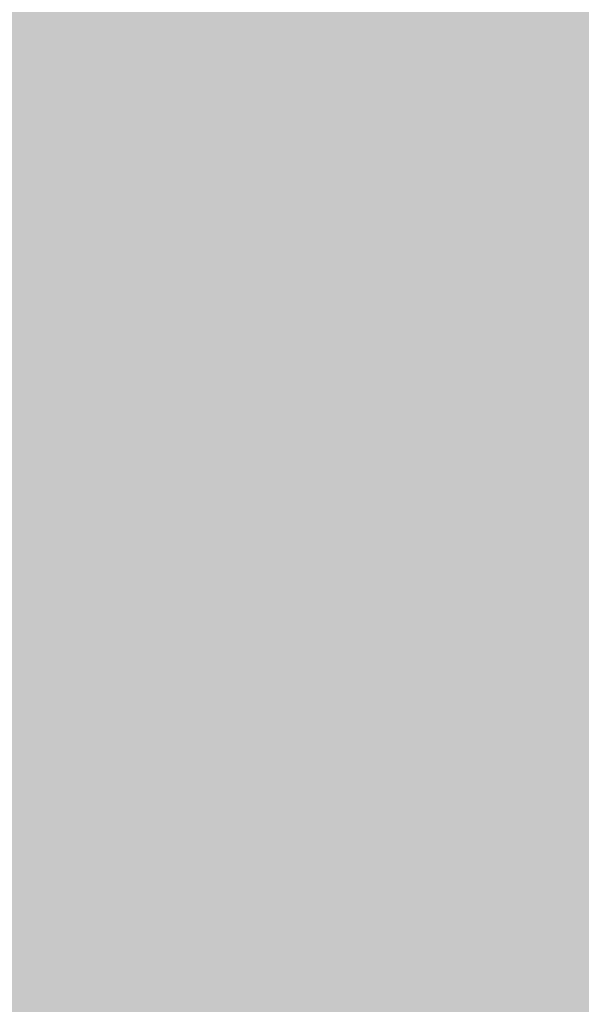
# Model space of a CAD drawing. Units: inches. Extents: x 2083 to 3317, y 1141 to 2115.
# Tile 171 of 256: x 3126.94671 to 3126.95594, y 1263.27402 to 1263.29018. Entities that reach past the tile are written whole.
import ezdxf

# ---------------------------------------------------------------- set-up
doc = ezdxf.new("R2010")
doc.units = ezdxf.units.IN
doc.layers.add('A-ANNO-DIMS', color=2, linetype='Continuous', lineweight=18)
doc.layers.add('A-WALL-PATT', color=251, linetype='Continuous', lineweight=13, true_color=0x636466)
doc.styles.get("Standard").update_dxf_attribs({"font": 'arial.ttf'})
doc.dimstyles.new('ISO-25', dxfattribs={"dimtxt": 12, "dimasz": 12, "dimexe": 1.25, "dimexo": 0.625, "dimtad": 1, "dimlunit": 3, "dimtxsty": 'Standard', "dimcen": 2.5, "dimadec": 0, "dimazin": 0, "dimtfac": 1, "dimtmove": 0, "dimatfit": 3, "dimfxl": 1, "dimarcsym": 0})

# ---------------------------------------------------------------- blocks, each defined once
blk = doc.blocks.new('*D26')
at = {"layer": 'A-ANNO-DIMS', "color": 0, "lineweight": -2, "transparency": 16777216}
for p, q in [((3088.985844, 1274.915092), (3088.985844, 1270.951963)), ((3111.240037, 1274.915092), (3111.240037, 1270.951963)), ((3076.985844, 1272.201963), (2840.262447, 1272.201963)), ((3111.240037, 1272.201963), (3088.985844, 1272.201963)), ((3123.240037, 1272.201963), (3135.240037, 1272.201963))]:
    blk.add_line(p, q, dxfattribs=at)
at = {"layer": 'A-ANNO-DIMS', "color": 0, "transparency": 16777216}
for points in [[(3076.985844, 1274.201963), (3076.985844, 1270.201963), (3088.985844, 1272.201963)], [(3123.240037, 1274.201963), (3123.240037, 1270.201963), (3111.240037, 1272.201963)]]:
    blk.add_solid(points, dxfattribs=at)
at = {"layer": 'Defpoints', "color": 0, "transparency": 16777216}
for p in [(3088.985844, 1275.540092), (3111.240037, 1275.540092), (3088.985844, 1272.201963)]:
    blk.add_point(p, dxfattribs=at)
at = {"layer": 'A-ANNO-DIMS', "color": 0, "transparency": 16777216, "insert": (2952.624146, 1279.031602), "char_height": 12, "attachment_point": 5}
blk.add_mtext('NIGHTSTAND 1\'-10 1/2" TYP.', dxfattribs=at)
blk = doc.blocks.new('*D27')
at = {"layer": 'A-ANNO-DIMS', "color": 0, "lineweight": -2, "transparency": 16777216}
for p, q in [((3114.578165, 1309.794285), (3114.578165, 1321.794285)), ((3111.865037, 1297.794285), (3115.828165, 1297.794285)), ((3114.578165, 1297.794285), (3114.578165, 1275.540092)), ((3111.865037, 1275.540092), (3115.828165, 1275.540092)), ((3114.578165, 1263.540092), (3114.578165, 1140.988591))]:
    blk.add_line(p, q, dxfattribs=at)
at = {"layer": 'A-ANNO-DIMS', "color": 0, "transparency": 16777216}
for points in [[(3112.578165, 1309.794285), (3116.578165, 1309.794285), (3114.578165, 1297.794285)], [(3112.578165, 1263.540092), (3116.578165, 1263.540092), (3114.578165, 1275.540092)]]:
    blk.add_solid(points, dxfattribs=at)
at = {"layer": 'Defpoints', "color": 0, "transparency": 16777216}
for p in [(3111.240037, 1297.794285), (3111.240037, 1275.540092), (3114.578165, 1275.540092)]:
    blk.add_point(p, dxfattribs=at)
at = {"layer": 'A-ANNO-DIMS', "color": 0, "transparency": 16777216, "insert": (3107.748527, 1196.264342), "char_height": 12, "attachment_point": 5, "rotation": 90}
blk.add_mtext('1\'-10 1/2" TYP.', dxfattribs=at)

msp = doc.modelspace()

# ---------------------------------------------------------------- hatches: boundary and pattern name
at = {"layer": 'A-WALL-PATT'}
h = msp.add_hatch(color=256, dxfattribs=at)
h.dxf.hatch_style = 1
h.paths.add_polyline_path([(3126.959783, 2020.76136), (2748.959783, 2020.76136), (2604.959783, 2020.76136), (2226.959783, 2020.76136), (2226.959783, 1702.76136), (2466.959783, 1702.76136), (2466.959783, 1582.76136), (2418.959783, 1582.76136), (2418.959783, 1477.76136), (2226.959783, 1477.76136), (2226.959783, 1263.26136), (2544.959783, 1263.26136), (2544.959783, 1411.76136), (2604.959783, 1411.76136), (2685.959783, 1411.76136), (2685.959783, 1420.76136), (2604.959783, 1420.76136), (2604.959783, 1573.76136), (2604.959783, 1702.76136), (2604.959783, 2011.76136), (2748.959783, 2011.76136), (2748.959783, 1702.76136), (2862.959783, 1702.76136), (2862.959783, 1621.76136), (2871.959783, 1621.76136), (2871.959783, 1702.76136), (2883.959783, 1702.76136), (2883.959783, 1706.939459, -0.026459), (2883.959783, 1711.76136), (2757.959783, 1711.76136), (2757.959783, 1807.76136), (2787.959783, 1807.76136), (2787.959783, 1812.26136), (2757.959783, 1812.26136), (2757.959783, 2011.76136), (2877.959783, 2011.76136), (2877.959783, 1812.26136), (2847.959783, 1812.26136), (2847.959783, 1807.76136), (2889.835742, 1807.76136), (2889.835742, 1812.26136), (2882.459783, 1812.26136), (2882.459783, 2011.76136), (3117.959783, 2011.76136), (3117.959783, 1812.26136), (2937.835742, 1812.26136), (2937.835742, 1807.76136), (2995.709783, 1807.76136), (2995.709783, 1796.117666), (3000.209783, 1796.117666), (3000.209783, 1807.76136), (3117.959783, 1807.76136), (3117.959783, 1711.76136), (3000.209783, 1711.76136), (3000.209783, 1760.117666), (2998.572705, 1760.117666, -0.020711), (2995.709783, 1760.117666), (2995.709783, 1711.76136), (2931.959783, 1711.76136), (2931.959783, 1702.76136), (3126.959783, 1702.76136)])
h.paths.add_polyline_path([(2471.459783, 2011.76136), (2471.459783, 1810.01136), (2462.716936, 1810.01136), (2462.716936, 1805.51136), (2505.959783, 1805.51136), (2505.959783, 1810.01136), (2475.959783, 1810.01136), (2475.959783, 2011.76136), (2595.959783, 2011.76136), (2595.959783, 1810.01136), (2565.959783, 1810.01136), (2565.959783, 1805.51136), (2595.959783, 1805.51136), (2595.959783, 1711.76136), (2235.959783, 1711.76136), (2235.959783, 1805.51136), (2353.709783, 1805.51136), (2353.709783, 1796.054162), (2358.209783, 1796.054162), (2358.209783, 1805.51136), (2414.716936, 1805.51136), (2414.716936, 1810.01136), (2235.959783, 1810.01136), (2235.959783, 2011.76136)], flags=16)
h.paths.add_polyline_path([(2270.204734, 1994.610008), (2270.204734, 1970.610008), (2246.204734, 1970.610008), (2246.204734, 1994.610008)], flags=0)
edge = h.paths.add_edge_path(flags=0)
edge.add_ellipse((2332.027391, 1899.798176), major_axis=(-3.042994, 3.042994), ratio=0.16825245, start_angle=-161.332166, end_angle=-156.307114, ccw=False)
edge.add_ellipse((2333.082037, 1898.74353), major_axis=(-1.054646, 1.054646), ratio=0.4535321, start_angle=-123.371019, end_angle=-94.159107)
edge = h.paths.add_edge_path(flags=0)
edge.add_ellipse((2332.027391, 1968.87629), major_axis=(3.042994, 3.042994), ratio=0.16825245, start_angle=18.667834, end_angle=23.692886)
edge.add_spline(control_points=[(2332.925596, 1970.691105), (2332.226768, 1970.3361), (2330.893709, 1969.658905), (2328.41308, 1970.932138), (2327.203934, 1967.748712), (2324.709596, 1969.955589), (2322.532822, 1967.012354), (2320.012846, 1971.295812), (2317.680308, 1968.157845), (2316.040526, 1967.102047), (2315.426904, 1966.809602)], knot_values=[0, 0, 0, 0, 2.267059, 4.324559, 6.685584, 8.878641, 11.121502, 14.300359, 17.755284, 19.732645, 19.732645, 19.732645, 19.732645], degree=3, periodic=0)
edge.add_ellipse((2332.027391, 1968.87629), major_axis=(3.042994, 3.042994), ratio=0.16825245, start_angle=18.667834, end_angle=23.692886, ccw=False)
edge.add_ellipse((2333.082037, 1969.930936), major_axis=(1.054646, 1.054646), ratio=0.4535321, start_angle=56.628981, end_angle=85.840893, ccw=False)
edge = h.paths.add_edge_path(flags=0)
edge.add_spline(control_points=[(2296.428287, 1967.987908), (2293.627804, 1965.336314), (2287.703624, 1959.727094), (2299.74386, 1949.995699), (2294.532591, 1935.668528), (2290.573228, 1920.603512), (2293.394124, 1909.973691), (2296.185407, 1904.966543)], knot_values=[0.099185, 0.099185, 0.099185, 0.099185, 0.345301, 0.619822, 0.982653, 1.386093, 1.810555, 1.810555, 1.810555, 1.810555], degree=3, periodic=0)
edge.add_spline(control_points=[(2296.185407, 1904.966543), (2297.383582, 1902.6193), (2298.000969, 1901.949312), (2298.55297, 1901.468155)], knot_values=[0.006246, 0.006246, 0.006246, 0.006246, 0.055476, 0.055476, 0.055476, 0.055476], degree=3, periodic=0)
edge.add_spline(control_points=[(2298.55297, 1901.468155), (2297.258612, 1900.923224), (2295.225294, 1900.232126), (2293.060229, 1900.614205), (2292.101423, 1900.788415), (2292.089578, 1900.790568)], knot_values=[0.312835, 0.312835, 0.312835, 0.312835, 0.40178, 0.474987, 0.475903, 0.475903, 0.475903, 0.475903], degree=3, periodic=0)
edge.add_arc((2292.793646, 1904.664109), 3.937008, 215.420897, 259.698179, ccw=False)
edge.add_spline(control_points=[(2289.585314, 1902.382304), (2289.476652, 1902.535087), (2289.36848, 1902.688035), (2289.260865, 1902.84117)], knot_values=[0.102872, 0.102872, 0.102872, 0.102872, 0.116896, 0.116896, 0.116896, 0.116896], degree=3, periodic=0)
edge.add_spline(control_points=[(2289.260865, 1902.84117), (2288.686604, 1902.550192), (2287.640048, 1902.019902), (2285.881337, 1901.873954), (2283.852972, 1901.504352), (2281.719987, 1899.710538), (2278.466991, 1899.492942), (2276.157136, 1901.883202), (2272.258953, 1899.804071), (2267.777605, 1901.843183), (2262.243882, 1900.184033), (2257.414927, 1901.782061), (2254.318374, 1900.72612), (2253.178285, 1900.337343)], knot_values=[0, 0, 0, 0, 1.907977, 3.477176, 5.261074, 7.972851, 11.680248, 13.717921, 16.939592, 22.789562, 27.502503, 33.595215, 37.145618, 37.145618, 37.145618, 37.145618], degree=3, periodic=0)
edge.add_line((2253.178285, 1900.337343), (2250.24424, 1902.84117))
edge.add_line((2250.24424, 1902.84117), (2250.24424, 1965.833296))
edge.add_line((2250.24424, 1965.833296), (2253.178285, 1968.337123))
edge.add_spline(control_points=[(2253.178285, 1968.337123), (2254.318374, 1967.948346), (2257.414927, 1966.892405), (2262.243882, 1968.490433), (2267.777605, 1966.831283), (2271.52673, 1968.537217), (2273.875914, 1967.828289), (2274.206701, 1967.727642)], knot_values=[0, 0, 0, 0, 0.09018, 0.244935, 0.364644, 0.513233, 0.537855, 0.537855, 0.537855, 0.537855], degree=3, periodic=0)
edge.add_arc((2274.352887, 1963.793349), 3.937008, 72.051134, 92.127949, ccw=False)
edge.add_arc((2281.296933, 1985.230003), 18.596298, 252.0511336, 288.5657217)
edge.add_arc((2292.316717, 1956.02888), 12.646081, 71.0267879, 113.7782184, ccw=False)
edge = h.paths.add_edge_path(flags=0)
edge.add_spline(control_points=[(2274.899415, 1951.856195), (2275.066156, 1951.616592), (2275.232687, 1951.376588), (2275.397987, 1951.135855)], knot_values=[1.409916, 1.409916, 1.409916, 1.409916, 1.43159, 1.43159, 1.43159, 1.43159], degree=3, periodic=0)
edge.add_spline(control_points=[(2275.397987, 1951.135855), (2275.792106, 1950.561885), (2276.179231, 1949.983774), (2276.545546, 1949.397103)], knot_values=[1.358238, 1.358238, 1.358238, 1.358238, 1.409916, 1.409916, 1.409916, 1.409916], degree=3, periodic=0)
edge.add_line((2276.545546, 1949.397103), (2277.437289, 1947.862185))
edge.add_spline(control_points=[(2277.437289, 1947.862185), (2276.303834, 1945.673115), (2274.639698, 1942.426882), (2274.631615, 1938.0939), (2272.799124, 1930.85155), (2274.356426, 1943.897046), (2275.947681, 1947.923356), (2276.545546, 1949.397103)], knot_values=[0.005632, 0.005632, 0.005632, 0.005632, 0.186014, 0.266002, 0.357087, 0.59639, 0.739732, 0.739732, 0.739732, 0.739732], degree=3, periodic=0)
edge.add_spline(control_points=[(2276.545546, 1949.397103), (2276.179231, 1949.983774), (2275.792106, 1950.561885), (2275.397987, 1951.135855)], knot_values=[1.358238, 1.358238, 1.358238, 1.358238, 1.409916, 1.409916, 1.409916, 1.409916], degree=3, periodic=0)
edge.add_spline(control_points=[(2275.397987, 1951.135855), (2274.9425, 1950.080452), (2274.20776, 1948.025272), (2273.934602, 1944.851477), (2272.468534, 1937.627489), (2273.466216, 1945.696466), (2274.700615, 1951.059472), (2274.899415, 1951.856195)], knot_values=[0.104364, 0.104364, 0.104364, 0.104364, 0.189636, 0.269624, 0.36071, 0.600013, 0.644622, 0.644622, 0.644622, 0.644622], degree=3, periodic=0)
h.paths.add_polyline_path([(2269.167514, 1963.127573, -0.357527), (2268.170633, 1960.97637, -0.092561), (2268.170633, 1939.436325, -0.357527), (2269.167514, 1937.285122, -0.357527), (2267.01631, 1938.282002, -0.164785), (2254.685581, 1938.282002, -0.357527), (2252.534378, 1937.285122, -0.357527), (2253.531259, 1939.436325, -0.092561), (2253.531259, 1960.97637, -0.357527), (2252.534378, 1963.127573, -0.357527), (2254.685581, 1962.130692, -0.164785), (2267.01631, 1962.130692, -0.357527)], flags=0)
h.paths.add_polyline_path([(2248.874068, 1967.8018), (2248.874068, 1957.02771), (2249.457783, 1957.02771), (2249.457783, 1911.646756), (2248.874068, 1911.646756), (2248.874068, 1900.872666), (2246.511863, 1900.872666, 0.197327), (2244.149658, 1902.456873), (2244.149658, 1966.217592, 0.197327), (2246.511863, 1967.8018)], flags=0)
h.paths.add_polyline_path([(2269.167514, 1931.389344, -0.357527), (2268.170633, 1929.238141, -0.092561), (2268.170633, 1907.698096, -0.357527), (2269.167514, 1905.546893, -0.357527), (2267.01631, 1906.543774, -0.164785), (2254.685581, 1906.543774, -0.357527), (2252.534378, 1905.546893, -0.357527), (2253.531259, 1907.698096, -0.092561), (2253.531259, 1929.238141, -0.357527), (2252.534378, 1931.389344, -0.357527), (2254.685581, 1930.392463, -0.164785), (2267.01631, 1930.392463, -0.357527)], flags=0)
edge = h.paths.add_edge_path(flags=0)
edge.add_spline(control_points=[(2276.196858, 1906.723702), (2276.168144, 1909.028928), (2276.114049, 1913.371852), (2270.598417, 1924.924978), (2273.905175, 1919.012779), (2275.921711, 1916.262063), (2275.47457, 1912.402149), (2277.257874, 1910.380621), (2276.696044, 1908.225036), (2276.646218, 1906.813023), (2276.617825, 1906.008407)], knot_values=[0, 0, 0, 0, 8.61026, 16.221274, 18.843057, 23.804898, 27.440828, 29.356102, 31.203478, 33.650687, 33.650687, 33.650687, 33.650687], degree=3, periodic=0)
edge.add_spline(control_points=[(2276.617825, 1906.008407), (2276.623313, 1905.624144), (2276.497738, 1904.628661), (2275.441779, 1903.854725), (2274.937314, 1903.08045), (2274.85908, 1902.84117)], knot_values=[0.156488, 0.156488, 0.156488, 0.156488, 0.184398, 0.231376, 0.250598, 0.250598, 0.250598, 0.250598], degree=3, periodic=0)
edge.add_line((2274.85908, 1902.84117), (2276.50598, 1902.84117))
edge.add_spline(control_points=[(2276.50598, 1902.84117), (2276.788308, 1903.08494), (2277.665071, 1904.125196), (2278.249538, 1904.340738), (2277.653872, 1908.527387), (2278.15567, 1906.227808), (2278.100464, 1905.285948), (2278.846675, 1904.069005), (2277.856785, 1903.414948), (2277.874191, 1902.99105), (2277.903562, 1902.84117)], knot_values=[0.059574, 0.059574, 0.059574, 0.059574, 0.080753, 0.103741, 0.16972, 0.176036, 0.207137, 0.240474, 0.262341, 0.27366, 0.27366, 0.27366, 0.27366], degree=3, periodic=0)
edge.add_line((2277.903562, 1902.84117), (2280.029825, 1902.84117))
edge.add_spline(control_points=[(2280.029825, 1902.84117), (2279.888221, 1903.088398), (2279.499257, 1903.981551), (2280.152284, 1905.939349), (2278.103615, 1909.657757), (2279.762395, 1907.185285), (2280.3279, 1904.874861), (2280.485109, 1903.48959), (2281.463269, 1903.249432), (2281.758343, 1902.936497), (2281.834036, 1902.84117)], knot_values=[0.013856, 0.013856, 0.013856, 0.013856, 0.034874, 0.088867, 0.107879, 0.126738, 0.158714, 0.193757, 0.217487, 0.226722, 0.226722, 0.226722, 0.226722], degree=3, periodic=0)
edge.add_spline(control_points=[(2281.834036, 1902.84117), (2281.787535, 1902.826703), (2281.647022, 1902.782988), (2281.395527, 1902.85949), (2281.088077, 1902.985242), (2280.720683, 1903.060902), (2280.333451, 1903.025726), (2280.124767, 1902.898879), (2280.029825, 1902.84117)], knot_values=[0, 0, 0, 0, 0.14413, 0.435517, 0.749276, 1.153046, 1.548371, 1.878348, 1.878348, 1.878348, 1.878348], degree=3, periodic=0)
edge.add_line((2280.029825, 1902.84117), (2277.903562, 1902.84117))
edge.add_spline(control_points=[(2277.903562, 1902.84117), (2277.892855, 1902.795855), (2277.865396, 1902.679637), (2277.607479, 1902.687483), (2277.27405, 1902.8007), (2276.837921, 1902.619775), (2276.583807, 1902.789261), (2276.50598, 1902.84117)], knot_values=[0, 0, 0, 0, 0.127189, 0.326199, 0.628009, 1.24357, 1.515331, 1.515331, 1.515331, 1.515331], degree=3, periodic=0)
edge.add_line((2276.50598, 1902.84117), (2274.85908, 1902.84117))
edge.add_spline(control_points=[(2274.85908, 1902.84117), (2274.814437, 1902.898587), (2274.72513, 1903.013446), (2274.493477, 1903.118968), (2274.244285, 1902.960539), (2273.937121, 1903.184942), (2273.614039, 1902.983143), (2273.408316, 1902.883045), (2273.322254, 1902.84117)], knot_values=[0, 0, 0, 0, 0.21843, 0.436957, 0.687977, 0.990379, 1.398396, 1.69185, 1.69185, 1.69185, 1.69185], degree=3, periodic=0)
edge.add_spline(control_points=[(2273.322254, 1902.84117), (2273.61674, 1903.445692), (2274.273998, 1904.538253), (2276.027239, 1904.573702), (2276.206963, 1906.583637), (2276.196858, 1906.723702)], knot_values=[0.012227, 0.012227, 0.012227, 0.012227, 0.059472, 0.106218, 0.134458, 0.134458, 0.134458, 0.134458], degree=3, periodic=0)
h.paths.add_polyline_path([(2270.776054, 1897.789828), (2270.776054, 1873.789828), (2246.776054, 1873.789828), (2246.776054, 1897.789828)], flags=0)
h.paths.add_polyline_path([(2353.709783, 1760.005059), (2353.709783, 1760.054162), (2358.209783, 1760.054162, -0.033729)], flags=0)
h.paths.add_polyline_path([(2321.819119, 1737.529186), (2341.995327, 1737.529186, -0.414214), (2343.203273, 1736.321241), (2343.203273, 1721.020596, -0.414214), (2341.995327, 1719.812651), (2321.819119, 1719.812651, -0.414214), (2320.611173, 1721.020596), (2320.611173, 1736.321241, -0.414214)], flags=0)
h.paths.add_polyline_path([(2324.23501, 1736.321241), (2339.579436, 1736.321241, -0.414214), (2341.995327, 1733.905349), (2341.995327, 1725.44973, -0.414214), (2339.579436, 1723.033839), (2333.680588, 1723.033839), (2333.845317, 1722.045467, -0.870646), (2335.425399, 1721.825893, -0.767327), (2333.922694, 1721.423245), (2331.291024, 1721.423245, -0.767327), (2329.788319, 1721.825893, -0.870646), (2331.368401, 1722.045467), (2331.53313, 1723.033839), (2324.23501, 1723.033839, -0.414214), (2321.819119, 1725.44973), (2321.819119, 1733.905349, -0.414214)], flags=0)
h.paths.add_polyline_path([(2570.483789, 1928.615444), (2589.683789, 1928.615444), (2590.168829, 1928.615444), (2590.168829, 1904.993397), (2570.483789, 1904.993397)], flags=0)
h.paths.add_polyline_path([(2574.447324, 1927.263822, -1), (2572.828836, 1927.263822, -1)], flags=0)
h.paths.add_polyline_path([(2573.089867, 1926.940877), (2573.925032, 1927.776042), (2574.147743, 1927.553332), (2573.312577, 1926.718166)], flags=0)
h.paths.add_polyline_path([(2578.779065, 1919.729618, -1), (2571.591663, 1919.729618, -1)], flags=0)
h.paths.add_polyline_path([(2578.385364, 1919.729618, -1), (2571.985364, 1919.729618, -1)], flags=0)
h.paths.add_polyline_path([(2331.595764, 1729.476216, -1), (2333.617954, 1729.476216, -1)], flags=0)
h.paths.add_polyline_path([(2578.034228, 1927.263822, -1), (2576.41574, 1927.263822, -1)], flags=0)
h.paths.add_polyline_path([(2576.688851, 1927.531089), (2576.911562, 1927.753799), (2577.746728, 1926.918634), (2577.524017, 1926.695923)], flags=0)
h.paths.add_polyline_path([(2578.139065, 1909.859539, -1), (2572.231663, 1909.859539, -1)], flags=0)
h.paths.add_polyline_path([(2577.745364, 1909.859539, -1), (2572.625364, 1909.859539, -1)], flags=0)
h.paths.add_polyline_path([(2583.797718, 1927.263822, -1), (2582.179229, 1927.263822, -1)], flags=0)
h.paths.add_polyline_path([(2582.718649, 1927.753799), (2583.553814, 1926.918634), (2583.331103, 1926.695923), (2582.495938, 1927.531089)], flags=0)
h.paths.add_polyline_path([(2582.495938, 1927.531089), (2582.718649, 1927.753799), (2583.553814, 1926.918634), (2583.331103, 1926.695923)], flags=0)
h.paths.add_polyline_path([(2587.739065, 1920.529618, -1), (2581.831663, 1920.529618, -1)], flags=0)
h.paths.add_polyline_path([(2587.345364, 1920.529618, -1), (2582.225364, 1920.529618, -1)], flags=0)
h.paths.add_polyline_path([(2587.384622, 1927.263822, -1), (2585.766133, 1927.263822, -1)], flags=0)
h.paths.add_polyline_path([(2586.081993, 1926.980247), (2586.917158, 1927.815412), (2587.139869, 1927.592702), (2586.304703, 1926.757536)], flags=0)
h.paths.add_polyline_path([(2588.379065, 1910.659539, -1), (2581.191663, 1910.659539, -1)], flags=0)
h.paths.add_polyline_path([(2587.985364, 1910.659539, -1), (2581.585364, 1910.659539, -1)], flags=0)
h.paths.add_polyline_path([(2417.167729, 1729.477895), (2437.343937, 1729.477895, -0.414214), (2438.551883, 1728.26995), (2438.551883, 1712.969306, -0.414214), (2437.343937, 1711.76136), (2417.167729, 1711.76136, -0.414214), (2415.959783, 1712.969306), (2415.959783, 1728.26995, -0.414214)], flags=0)
h.paths.add_polyline_path([(2419.58362, 1728.26995), (2434.928046, 1728.26995, -0.414214), (2437.343937, 1725.854059), (2437.343937, 1717.39844, -0.414214), (2434.928046, 1714.982548), (2429.029199, 1714.982548), (2429.193927, 1713.994176, -0.870646), (2430.774009, 1713.774603, -0.767327), (2429.271304, 1713.371954), (2426.639634, 1713.371954, -0.767327), (2425.136929, 1713.774603, -0.870646), (2426.717011, 1713.994176), (2426.88174, 1714.982548), (2419.58362, 1714.982548, -0.414214), (2417.167729, 1717.39844), (2417.167729, 1725.854059, -0.414214)], flags=0)
h.paths.add_polyline_path([(2419.58362, 1728.26995), (2434.928046, 1728.26995, -0.414214), (2437.343937, 1725.854059), (2437.343937, 1717.39844, -0.414214), (2434.928046, 1714.982548), (2429.029199, 1714.982548), (2428.358118, 1719.009034), (2427.552821, 1719.009034), (2426.88174, 1714.982548), (2419.58362, 1714.982548, -0.414214), (2417.167729, 1717.39844), (2417.167729, 1725.854059, -0.414214)], flags=0)
h.paths.add_polyline_path([(2426.944374, 1721.424925, -1), (2428.966564, 1721.424925, -1)], flags=0)
h.paths.add_polyline_path([(2475.959783, 1702.76136), (2595.959783, 1702.76136), (2595.959783, 1582.76136), (2475.959783, 1582.76136)], flags=16)
h.paths.add_polyline_path([(2427.959783, 1573.76136), (2595.959783, 1573.76136), (2595.959783, 1468.76136), (2595.959783, 1420.76136), (2384.459783, 1420.76136), (2384.459783, 1468.76136), (2427.959783, 1468.76136)], flags=16)
h.paths.add_polyline_path([(2379.959783, 1468.76136), (2379.959783, 1420.76136), (2235.959783, 1420.76136), (2235.959783, 1468.76136)], flags=16)
h.paths.add_polyline_path([(2317.815996, 1466.695767), (2337.992205, 1466.695767, -0.414214), (2339.20015, 1465.487821), (2339.20015, 1450.187177, -0.414214), (2337.992205, 1448.979232), (2317.815996, 1448.979232, -0.414214), (2316.608051, 1450.187177), (2316.608051, 1465.487821, -0.414214)], flags=0)
h.paths.add_polyline_path([(2320.231887, 1465.487821), (2335.576313, 1465.487821, -0.414214), (2337.992205, 1463.07193), (2337.992205, 1454.616311, -0.414214), (2335.576313, 1452.20042), (2329.677466, 1452.20042), (2329.842195, 1451.212047, -0.870646), (2331.422276, 1450.992474, -0.767327), (2329.919571, 1450.589826), (2327.287902, 1450.589826, -0.767327), (2325.785197, 1450.992474, -0.870646), (2327.365278, 1451.212047), (2327.530007, 1452.20042), (2320.231887, 1452.20042, -0.414214), (2317.815996, 1454.616311), (2317.815996, 1463.07193, -0.414214)], flags=0)
h.paths.add_polyline_path([(2320.231887, 1465.487821), (2335.576313, 1465.487821, -0.414214), (2337.992205, 1463.07193), (2337.992205, 1454.616311, -0.414214), (2335.576313, 1452.20042), (2329.677466, 1452.20042), (2329.006385, 1456.226905), (2328.201088, 1456.226905), (2327.530007, 1452.20042), (2320.231887, 1452.20042, -0.414214), (2317.815996, 1454.616311), (2317.815996, 1463.07193, -0.414214)], flags=0)
h.paths.add_polyline_path([(2327.592641, 1458.642796, -1), (2329.614832, 1458.642796, -1)], flags=0)
h.paths.add_polyline_path([(2244.411744, 1433.340453), (2241.920945, 1433.340453, -0.414214), (2240.017856, 1435.243542), (2240.017856, 1440.952808, -0.414211), (2241.920925, 1442.855897), (2244.411744, 1442.855897, -1.976472)], flags=0)
h.paths.add_polyline_path([(2245.356888, 1434.397536, -0.414214), (2245.356888, 1441.798814, -2.144098)], flags=0)
h.paths.add_polyline_path([(2535.959783, 1416.26136), (2535.959783, 1272.26136), (2235.959783, 1272.26136), (2235.959783, 1416.26136)], flags=16)
h.paths.add_polyline_path([(2260.119561, 1384.292841), (2260.119561, 1362.038649), (2237.865369, 1362.038649), (2237.865369, 1384.292841)], flags=0)
edge = h.paths.add_edge_path(flags=0)
edge.add_line((2318.251847, 1362.093298), (2318.145797, 1362.000973))
edge.add_ellipse((2317.445116, 1360.431044), major_axis=(2.82164, 2.82164), ratio=0.16825245, start_angle=18.667834, end_angle=20.948127, ccw=False)
edge.add_ellipse((2318.423045, 1361.408974), major_axis=(0.977929, 0.977929), ratio=0.4535321, start_angle=56.628981, end_angle=70.226201, ccw=False)
edge = h.paths.add_edge_path(flags=0)
edge.add_line((2319.10737, 1295.571078), (2319.015044, 1295.677128))
edge.add_ellipse((2317.445116, 1296.377809), major_axis=(-2.82164, 2.82164), ratio=0.16825245, start_angle=-161.332166, end_angle=-159.051873, ccw=False)
edge.add_ellipse((2318.423045, 1295.39988), major_axis=(-0.977929, 0.977929), ratio=0.4535321, start_angle=-123.371019, end_angle=-109.773799)
edge = h.paths.add_edge_path(flags=0)
edge.add_spline(control_points=[(2284.210349, 1301.170219), (2284.580688, 1300.444719), (2284.891189, 1299.892024), (2285.159553, 1299.461018)], knot_values=[0.039066, 0.039066, 0.039066, 0.039066, 0.055476, 0.055476, 0.055476, 0.055476], degree=3, periodic=0)
edge.add_line((2285.159553, 1299.461018), (2284.210349, 1301.170219))
edge = h.paths.add_edge_path(flags=0)
edge.add_line((2280.412458, 1297.298013), (2283.369991, 1297.036122))
edge.add_line((2283.369991, 1297.036122), (2286.40569, 1297.92631))
edge.add_spline(control_points=[(2286.40569, 1297.92631), (2285.305487, 1297.463119), (2284.344777, 1297.129151), (2283.369991, 1297.036122)], knot_values=[0.394369, 0.394369, 0.394369, 0.394369, 0.475903, 0.475903, 0.475903, 0.475903], degree=3, periodic=0)
edge.add_spline(control_points=[(2283.369991, 1297.036122), (2283.28139, 1297.027666), (2282.316289, 1296.957336), (2281.312502, 1297.134479), (2280.423441, 1297.296016), (2280.412458, 1297.298013)], knot_values=[0.312835, 0.312835, 0.312835, 0.312835, 0.320246, 0.393453, 0.394369, 0.394369, 0.394369, 0.394369], degree=3, periodic=0)
edge = h.paths.add_edge_path(flags=0)
edge.add_line((2284.435561, 1359.607285), (2280.446291, 1355.328047))
edge.add_line((2280.446291, 1355.328047), (2279.579987, 1351.017754))
edge.add_line((2279.579987, 1351.017754), (2282.412974, 1346.580433))
edge.add_spline(control_points=[(2282.412974, 1346.580433), (2283.153331, 1345.589236), (2284.252896, 1344.028897), (2284.801037, 1342.387167), (2284.935162, 1341.805544)], knot_values=[1.240098, 1.240098, 1.240098, 1.240098, 1.332892, 1.382712, 1.382712, 1.382712, 1.382712], degree=3, periodic=0)
edge.add_spline(control_points=[(2284.935162, 1341.805544), (2285.319108, 1340.1406), (2285.233029, 1338.409204), (2284.909938, 1336.654122)], knot_values=[1.097484, 1.097484, 1.097484, 1.097484, 1.240098, 1.240098, 1.240098, 1.240098], degree=3, periodic=0)
edge.add_spline(control_points=[(2284.909938, 1336.654122), (2284.586848, 1334.89904), (2284.026745, 1333.120272), (2283.462644, 1331.360585)], knot_values=[0.95487, 0.95487, 0.95487, 0.95487, 1.097484, 1.097484, 1.097484, 1.097484], degree=3, periodic=0)
edge.add_line((2283.462644, 1331.360585), (2281.890376, 1326.153357))
edge.add_line((2281.890376, 1326.153357), (2280.756259, 1321.056089))
edge.add_line((2280.756259, 1321.056089), (2280.299205, 1316.001977))
edge.add_line((2280.299205, 1316.001977), (2280.715933, 1310.950068))
edge.add_line((2280.715933, 1310.950068), (2282.028094, 1305.972137))
edge.add_line((2282.028094, 1305.972137), (2284.210349, 1301.170219))
edge.add_spline(control_points=[(2284.210349, 1301.170219), (2283.340731, 1302.730185), (2282.611904, 1304.336493), (2282.028094, 1305.972137)], knot_values=[0.099185, 0.099185, 0.099185, 0.099185, 0.241799, 0.241799, 0.241799, 0.241799], degree=3, periodic=0)
edge.add_spline(control_points=[(2282.028094, 1305.972137), (2281.444283, 1307.60778), (2281.005489, 1309.272759), (2280.715933, 1310.950068)], knot_values=[0.241799, 0.241799, 0.241799, 0.241799, 0.384413, 0.384413, 0.384413, 0.384413], degree=3, periodic=0)
edge.add_spline(control_points=[(2280.715933, 1310.950068), (2280.433241, 1312.587613), (2280.289386, 1314.276959), (2280.298894, 1315.962032), (2280.299205, 1316.001977)], knot_values=[0.384413, 0.384413, 0.384413, 0.384413, 0.523647, 0.527028, 0.527028, 0.527028, 0.527028], degree=3, periodic=0)
edge.add_spline(control_points=[(2280.299205, 1316.001977), (2280.312326, 1317.686955), (2280.477871, 1319.367926), (2280.756259, 1321.056089)], knot_values=[0.527028, 0.527028, 0.527028, 0.527028, 0.669642, 0.669642, 0.669642, 0.669642], degree=3, periodic=0)
edge.add_spline(control_points=[(2280.756259, 1321.056089), (2281.034648, 1322.744252), (2281.42588, 1324.439608), (2281.890376, 1326.153357)], knot_values=[0.669642, 0.669642, 0.669642, 0.669642, 0.812256, 0.812256, 0.812256, 0.812256], degree=3, periodic=0)
edge.add_spline(control_points=[(2281.890376, 1326.153357), (2282.264383, 1327.533251), (2282.78787, 1329.26181), (2283.352751, 1331.01778), (2283.462644, 1331.360585)], knot_values=[0.812256, 0.812256, 0.812256, 0.812256, 0.927087, 0.95487, 0.95487, 0.95487, 0.95487], degree=3, periodic=0)
edge.add_line((2283.462644, 1331.360585), (2284.909938, 1336.654122))
edge.add_line((2284.909938, 1336.654122), (2284.935162, 1341.805544))
edge.add_line((2284.935162, 1341.805544), (2282.412974, 1346.580433))
edge.add_spline(control_points=[(2282.412974, 1346.580433), (2281.275127, 1348.103792), (2280.078447, 1349.570318), (2279.579987, 1351.017754)], knot_values=[1.382712, 1.382712, 1.382712, 1.382712, 1.525326, 1.525326, 1.525326, 1.525326], degree=3, periodic=0)
edge.add_spline(control_points=[(2279.579987, 1351.017754), (2279.443282, 1351.414721), (2279.136312, 1352.856922), (2279.73519, 1354.290385), (2280.446291, 1355.328047)], knot_values=[1.525326, 1.525326, 1.525326, 1.525326, 1.564439, 1.667941, 1.667941, 1.667941, 1.667941], degree=3, periodic=0)
edge.add_spline(control_points=[(2280.446291, 1355.328047), (2281.426113, 1356.757835), (2282.930837, 1358.18256), (2284.435561, 1359.607285)], knot_values=[1.667941, 1.667941, 1.667941, 1.667941, 1.810555, 1.810555, 1.810555, 1.810555], degree=3, periodic=0)
edge.add_arc((2280.623075, 1348.518181), 11.72618, 71.0267879, 113.7782184)
edge.add_arc((2270.404892, 1375.595156), 17.243567, 252.0511336, 288.5657217, ccw=False)
edge.add_arc((2263.965969, 1355.717847), 3.650622, 72.051134, 92.127949)
edge.add_arc((2263.965969, 1355.717847), 3.650622, 92.127949, 177.98513)
edge.add_spline(control_points=[(2260.317604, 1355.846199), (2260.260417, 1354.220668), (2260.551278, 1350.186547), (2262.999344, 1346.766251), (2264.472741, 1344.649024)], knot_values=[1.43159, 1.43159, 1.43159, 1.43159, 1.564144, 1.770695, 1.770695, 1.770695, 1.770695], degree=3, periodic=0)
edge.add_line((2264.472741, 1344.649024), (2264.93559, 1343.98253))
edge.add_spline(control_points=[(2263.801044, 1340.248105), (2263.843238, 1340.514088), (2264.067244, 1341.756465), (2264.512693, 1343.002453), (2264.935047, 1343.981083)], knot_values=[0.53657, 0.53657, 0.53657, 0.53657, 0.559349, 0.644622, 0.644622, 0.644622, 0.644622], degree=3, periodic=0)
edge.add_spline(control_points=[(2264.935047, 1343.981083), (2265.117771, 1343.714975), (2265.298875, 1343.447906), (2265.476756, 1343.179365)], knot_values=[1.384077, 1.384077, 1.384077, 1.384077, 1.409916, 1.409916, 1.409916, 1.409916], degree=3, periodic=0)
edge.add_spline(control_points=[(2265.476756, 1343.179365), (2265.654637, 1342.910823), (2265.829296, 1342.64081), (2265.99913, 1342.368812)], knot_values=[1.358238, 1.358238, 1.358238, 1.358238, 1.384077, 1.384077, 1.384077, 1.384077], degree=3, periodic=0)
edge.add_line((2265.99913, 1342.368812), (2266.826006, 1340.945547))
edge.add_spline(control_points=[(2266.826006, 1340.945547), (2268.894401, 1337.089691), (2271.398173, 1325.843001), (2270.516164, 1310.568557), (2275.919376, 1301.860609), (2277.789511, 1299.19945)], knot_values=[0.116896, 0.116896, 0.116896, 0.116896, 0.472987, 1.050969, 1.313793, 1.313793, 1.313793, 1.313793], degree=3, periodic=0)
edge.add_spline(control_points=[(2277.789511, 1299.19945), (2277.839405, 1299.128452), (2277.889428, 1299.057498), (2277.939572, 1298.986584)], knot_values=[0.109884, 0.109884, 0.109884, 0.109884, 0.116896, 0.116896, 0.116896, 0.116896], degree=3, periodic=0)
edge.add_line((2277.939572, 1298.986584), (2277.788849, 1299.199114))
edge.add_spline(control_points=[(2277.788849, 1299.199114), (2277.256582, 1298.929414), (2276.28635, 1298.437902), (2275.039352, 1298.334419), (2274.38333, 1298.238895), (2274.215254, 1298.209338)], knot_values=[33.12187, 33.12187, 33.12187, 33.12187, 35.029056, 36.598255, 37.144827, 37.144827, 37.144827, 37.144827], degree=3, periodic=0)
edge.add_line((2274.215254, 1298.209338), (2273.073147, 1297.892961))
edge.add_spline(control_points=[(2273.073147, 1297.892961), (2272.322936, 1297.579784), (2271.039151, 1296.510508), (2269.248395, 1296.226062), (2268.4231, 1296.374654)], knot_values=[26.532584, 26.532584, 26.532584, 26.532584, 29.198919, 31.839101, 31.839101, 31.839101, 31.839101], degree=3, periodic=0)
edge.add_line((2268.4231, 1296.374654), (2263.878501, 1297.457534))
edge.add_spline(control_points=[(2263.878501, 1297.457534), (2263.556077, 1297.359435), (2261.860306, 1296.838694), (2260.23878, 1297.282407), (2258.933454, 1297.516461)], knot_values=[15.919551, 15.919551, 15.919551, 15.919551, 16.939592, 21.226067, 21.226067, 21.226067, 21.226067], degree=3, periodic=0)
edge.add_line((2258.933454, 1297.516461), (2254.055233, 1297.32901))
edge.add_spline(control_points=[(2254.055233, 1297.32901), (2253.755525, 1297.295815), (2252.113683, 1297.165174), (2250.461869, 1297.544221), (2249.129686, 1297.667882)], knot_values=[5.306517, 5.306517, 5.306517, 5.306517, 6.276435, 10.613034, 10.613034, 10.613034, 10.613034], degree=3, periodic=0)
edge.add_line((2249.129686, 1297.667882), (2244.33165, 1296.877756))
edge.add_line((2244.33165, 1296.877756), (2241.611033, 1299.19945))
edge.add_line((2241.611033, 1299.19945), (2241.611033, 1357.609404))
edge.add_line((2241.611033, 1357.609404), (2244.33165, 1359.931097))
edge.add_line((2244.33165, 1359.931097), (2252.728823, 1359.542692))
edge.add_spline(control_points=[(2252.728823, 1359.542692), (2252.870939, 1359.54644), (2253.30574, 1359.548172), (2253.739845, 1359.514274), (2254.031742, 1359.482426)], knot_values=[0.233291, 0.233291, 0.233291, 0.233291, 0.244935, 0.268927, 0.268927, 0.268927, 0.268927], degree=3, periodic=0)
edge.add_line((2254.031742, 1359.482426), (2259.58719, 1359.41639))
edge.add_spline(control_points=[(2259.58719, 1359.41639), (2260.677068, 1359.628503), (2262.073197, 1359.897003), (2263.523692, 1359.459278), (2263.830417, 1359.365952)], knot_values=[0.422516, 0.422516, 0.422516, 0.422516, 0.513233, 0.537855, 0.537855, 0.537855, 0.537855], degree=3, periodic=0)
edge.add_arc((2263.965969, 1355.717847), 3.650622, 72.051134, 92.127949, ccw=False)
edge.add_arc((2270.404892, 1375.595156), 17.243567, 252.0511336, 288.5657217)
edge.add_arc((2280.623075, 1348.518181), 11.72618, 71.0267879, 113.7782184, ccw=False)
h.paths.add_polyline_path([(2240.34053, 1359.434715), (2240.34053, 1349.444353), (2240.881785, 1349.444353), (2240.881785, 1307.3645), (2240.34053, 1307.3645), (2240.34053, 1297.374138), (2238.150157, 1297.374138, 0.197327), (2235.959783, 1298.843108), (2235.959783, 1357.965746, 0.197327), (2238.150157, 1359.434715)], flags=0)
h.paths.add_polyline_path([(2259.15779, 1355.1005, -0.357527), (2258.233425, 1353.10578, -0.092561), (2258.233425, 1333.132601, -0.357527), (2259.15779, 1331.13788, -0.357527), (2257.16307, 1332.062246, -0.164785), (2245.729302, 1332.062246, -0.357527), (2243.734582, 1331.13788, -0.357527), (2244.658947, 1333.132601, -0.092561), (2244.658947, 1353.10578, -0.357527), (2243.734582, 1355.1005, -0.357527), (2245.729302, 1354.176135, -0.164785), (2257.16307, 1354.176135, -0.357527)], flags=0)
edge = h.paths.add_edge_path(flags=0)
edge.add_line((2265.99913, 1342.368812), (2266.826006, 1340.945547))
edge.add_line((2266.826006, 1340.945547), (2265.307557, 1337.814066))
edge.add_line((2265.307557, 1337.814066), (2264.358232, 1334.652939))
edge.add_line((2264.358232, 1334.652939), (2264.262012, 1333.799705))
edge.add_spline(control_points=[(2264.262012, 1333.799705), (2264.208357, 1333.187055), (2264.16206, 1332.365525), (2264.007144, 1331.413933), (2263.969049, 1331.201834)], knot_values=[0.464444, 0.464444, 0.464444, 0.464444, 0.516691, 0.531608, 0.531608, 0.531608, 0.531608], degree=3, periodic=0)
edge.add_spline(control_points=[(2263.969049, 1331.201834), (2263.774535, 1330.118873), (2263.42437, 1328.790839), (2263.25742, 1328.530652), (2263.234028, 1328.514612)], knot_values=[0.372682, 0.372682, 0.372682, 0.372682, 0.44885, 0.464444, 0.464444, 0.464444, 0.464444], degree=3, periodic=0)
edge.add_spline(control_points=[(2263.234028, 1328.514612), (2263.096382, 1328.420227), (2263.13117, 1329.301477), (2263.274953, 1330.615749)], knot_values=[0.280919, 0.280919, 0.280919, 0.280919, 0.372682, 0.372682, 0.372682, 0.372682], degree=3, periodic=0)
edge.add_spline(control_points=[(2263.274953, 1330.615749), (2263.418736, 1331.930022), (2263.671515, 1333.677318), (2263.969852, 1335.315027)], knot_values=[0.189157, 0.189157, 0.189157, 0.189157, 0.280919, 0.280919, 0.280919, 0.280919], degree=3, periodic=0)
edge.add_spline(control_points=[(2263.969852, 1335.315027), (2264.100496, 1336.032192), (2264.418783, 1337.621911), (2264.754848, 1338.86443), (2264.947419, 1339.491124)], knot_values=[0.097394, 0.097394, 0.097394, 0.097394, 0.137578, 0.189157, 0.189157, 0.189157, 0.189157], degree=3, periodic=0)
edge.add_spline(control_points=[(2264.947419, 1339.491124), (2265.290017, 1340.606055), (2265.644238, 1341.493996), (2265.99913, 1342.368812)], knot_values=[0.005632, 0.005632, 0.005632, 0.005632, 0.097394, 0.097394, 0.097394, 0.097394], degree=3, periodic=0)
h.paths.add_polyline_path([(2259.15779, 1325.670973, -0.357527), (2258.233425, 1323.676253, -0.092561), (2258.233425, 1303.703073, -0.357527), (2259.15779, 1301.708353, -0.357527), (2257.16307, 1302.632719, -0.164785), (2245.729302, 1302.632719, -0.357527), (2243.734582, 1301.708353, -0.357527), (2244.658947, 1303.703073, -0.092561), (2244.658947, 1323.676253, -0.357527), (2243.734582, 1325.670973, -0.357527), (2245.729302, 1324.746608, -0.164785), (2257.16307, 1324.746608, -0.357527)], flags=0)
edge = h.paths.add_edge_path(flags=0)
edge.add_spline(control_points=[(2261.708938, 1317.311421), (2261.679482, 1317.41758), (2261.761858, 1317.388535), (2262.490736, 1316.089873), (2262.962185, 1315.300897)], knot_values=[14.955861, 14.955861, 14.955861, 14.955861, 16.221274, 18.694826, 18.694826, 18.694826, 18.694826], degree=3, periodic=0)
edge.add_spline(control_points=[(2262.962185, 1315.300897), (2262.990437, 1315.253617), (2263.702096, 1314.067376), (2264.348983, 1313.127153), (2264.730054, 1312.164154)], knot_values=[18.694826, 18.694826, 18.694826, 18.694826, 18.843057, 22.433791, 22.433791, 22.433791, 22.433791], degree=3, periodic=0)
edge.add_spline(control_points=[(2264.730054, 1312.164154), (2264.875565, 1311.796437), (2265.176873, 1310.769807), (2265.143069, 1309.559262), (2265.247736, 1308.824193)], knot_values=[22.433791, 22.433791, 22.433791, 22.433791, 23.804898, 26.172756, 26.172756, 26.172756, 26.172756], degree=3, periodic=0)
edge.add_line((2265.247736, 1308.824193), (2265.850774, 1307.171888))
edge.add_spline(control_points=[(2265.850774, 1307.171888), (2266.065025, 1306.821678), (2266.384387, 1306.332246), (2266.4244, 1305.780549), (2266.420369, 1305.611216)], knot_values=[28.062562, 28.062562, 28.062562, 28.062562, 29.356102, 29.911721, 29.911721, 29.911721, 29.911721], degree=3, periodic=0)
edge.add_spline(control_points=[(2266.420369, 1305.611216), (2266.416116, 1305.43259), (2266.393999, 1305.249998), (2266.364777, 1305.065857)], knot_values=[29.911721, 29.911721, 29.911721, 29.911721, 30.497837, 30.497837, 30.497837, 30.497837], degree=3, periodic=0)
edge.add_line((2266.364777, 1305.065857), (2266.066151, 1302.136295))
edge.add_spline(control_points=[(2266.066151, 1302.136295), (2266.07124, 1301.779984), (2265.998076, 1301.199985), (2265.663266, 1300.758961), (2265.508908, 1300.585882)], knot_values=[0.156488, 0.156488, 0.156488, 0.156488, 0.184398, 0.203543, 0.203543, 0.203543, 0.203543], degree=3, periodic=0)
edge.add_line((2265.508908, 1300.585882), (2264.435341, 1299.19945))
edge.add_line((2264.435341, 1299.19945), (2265.962442, 1299.19945))
edge.add_line((2265.962442, 1299.19945), (2267.33599, 1301.175276))
edge.add_line((2267.33599, 1301.175276), (2267.311667, 1301.986237))
edge.add_spline(control_points=[(2267.311667, 1301.986237), (2267.261111, 1302.862396), (2267.160212, 1303.737132), (2267.271486, 1303.325896)], knot_values=[0.126229, 0.126229, 0.126229, 0.126229, 0.166617, 0.166617, 0.166617, 0.166617], degree=3, periodic=0)
edge.add_spline(control_points=[(2267.271486, 1303.325896), (2267.280035, 1303.294305), (2267.309785, 1303.175366), (2267.37345, 1302.883608), (2267.406123, 1302.682829), (2267.417926, 1302.601025)], knot_values=[0.166617, 0.166617, 0.166617, 0.166617, 0.16972, 0.176036, 0.180765, 0.180765, 0.180765, 0.180765], degree=3, periodic=0)
edge.add_spline(control_points=[(2267.743891, 1300.987505), (2267.687583, 1301.150943), (2267.48052, 1301.656664), (2267.483751, 1302.144788), (2267.417926, 1302.601025)], knot_values=[0.180765, 0.180765, 0.180765, 0.180765, 0.193767, 0.220139, 0.220139, 0.220139, 0.220139], degree=3, periodic=0)
edge.add_line((2267.417926, 1302.601025), (2267.743891, 1300.987505))
edge.add_spline(control_points=[(2267.743891, 1300.987505), (2267.831961, 1300.731878), (2267.932021, 1300.309904), (2267.554841, 1299.974518), (2267.429366, 1299.829207)], knot_values=[0.220139, 0.220139, 0.220139, 0.220139, 0.240474, 0.25489, 0.25489, 0.25489, 0.25489], degree=3, periodic=0)
edge.add_line((2267.429366, 1299.829207), (2267.258361, 1299.19945))
edge.add_line((2267.258361, 1299.19945), (2269.229956, 1299.19945))
edge.add_spline(control_points=[(2269.229956, 1299.19945), (2269.098653, 1299.428694), (2268.842774, 1300.016251), (2269.011575, 1300.915923), (2268.946796, 1301.66074)], knot_values=[0.013856, 0.013856, 0.013856, 0.013856, 0.034874, 0.067073, 0.067073, 0.067073, 0.067073], degree=3, periodic=0)
edge.add_line((2268.946796, 1301.66074), (2268.431582, 1303.603109))
edge.add_spline(control_points=[(2268.431582, 1303.603109), (2268.175596, 1304.192375), (2267.596214, 1305.251298), (2268.040698, 1304.62321), (2268.251394, 1304.282421)], knot_values=[0.090155, 0.090155, 0.090155, 0.090155, 0.107879, 0.120289, 0.120289, 0.120289, 0.120289], degree=3, periodic=0)
edge.add_spline(control_points=[(2268.251394, 1304.282421), (2268.360882, 1304.105329), (2269.057753, 1302.917983), (2269.382691, 1301.590419), (2269.521405, 1300.775931), (2269.57522, 1300.555784)], knot_values=[0.120289, 0.120289, 0.120289, 0.120289, 0.126738, 0.158714, 0.173506, 0.173506, 0.173506, 0.173506], degree=3, periodic=0)
edge.add_line((2269.57522, 1300.555784), (2270.685798, 1299.421258))
edge.add_spline(control_points=[(2270.685798, 1299.421258), (2270.767221, 1299.357251), (2270.837852, 1299.281401), (2270.902925, 1299.19945)], knot_values=[0.21816, 0.21816, 0.21816, 0.21816, 0.226722, 0.226722, 0.226722, 0.226722], degree=3, periodic=0)
edge.add_line((2270.937201, 1299.192913), (2270.902925, 1299.19945))
edge.add_spline(control_points=[(2270.902925, 1299.19945), (2270.859806, 1299.186035), (2270.729515, 1299.1455), (2270.496314, 1299.216437), (2270.271661, 1299.308323), (2270.121017, 1299.347961), (2270.063339, 1299.359557)], knot_values=[0.939174, 0.939174, 0.939174, 0.939174, 1.083304, 1.374691, 1.68845, 1.878348, 1.878348, 1.878348, 1.878348], degree=3, periodic=0)
edge.add_line((2270.063339, 1299.359557), (2269.229956, 1299.19945))
edge.add_line((2269.229956, 1299.19945), (2267.258361, 1299.19945))
edge.add_spline(control_points=[(2267.258361, 1299.19945), (2267.248433, 1299.157431), (2267.222971, 1299.049667), (2266.983816, 1299.056942), (2266.80921, 1299.11623), (2266.676905, 1299.109091), (2266.636531, 1299.104815)], knot_values=[0.757665, 0.757665, 0.757665, 0.757665, 0.884854, 1.083864, 1.385675, 1.515331, 1.515331, 1.515331, 1.515331], degree=3, periodic=0)
edge.add_spline(control_points=[(2266.636531, 1299.104815), (2266.485225, 1299.088788), (2266.235807, 1299.017123), (2266.034608, 1299.151317), (2265.962442, 1299.19945)], knot_values=[0, 0, 0, 0, 0.485905, 0.757665, 0.757665, 0.757665, 0.757665], degree=3, periodic=0)
edge.add_line((2265.962442, 1299.19945), (2264.435341, 1299.19945))
edge.add_line((2264.435341, 1299.19945), (2263.858444, 1299.367118))
edge.add_spline(control_points=[(2263.858444, 1299.367118), (2263.818943, 1299.370905), (2263.779528, 1299.385721), (2263.740131, 1299.401504)], knot_values=[0.845925, 0.845925, 0.845925, 0.845925, 0.978627, 0.978627, 0.978627, 0.978627], degree=3, periodic=0)
edge.add_line((2263.721786, 1299.396425), (2263.010306, 1299.19945))
edge.add_spline(control_points=[(2263.010306, 1299.19945), (2263.245794, 1299.682859), (2263.506032, 1300.128107), (2263.873494, 1300.408028)], knot_values=[0.012227, 0.012227, 0.012227, 0.012227, 0.052971, 0.052971, 0.052971, 0.052971], degree=3, periodic=0)
edge.add_spline(control_points=[(2263.873494, 1300.408028), (2263.932131, 1300.452695), (2264.084243, 1300.552979), (2264.255189, 1300.624223), (2264.359686, 1300.664747)], knot_values=[0.052971, 0.052971, 0.052971, 0.052971, 0.059472, 0.069086, 0.069086, 0.069086, 0.069086], degree=3, periodic=0)
edge.add_line((2264.359686, 1300.664747), (2265.1419, 1301.077774))
edge.add_line((2265.1419, 1301.077774), (2265.675806, 1302.799558))
edge.add_line((2265.675806, 1302.799558), (2265.5407, 1305.704066))
edge.add_line((2265.5407, 1305.704066), (2264.803073, 1309.327724))
edge.add_line((2264.803073, 1309.327724), (2263.040535, 1314.091791))
edge.add_spline(control_points=[(2263.040535, 1314.091791), (2262.383572, 1315.671438), (2261.795972, 1316.997749), (2261.708938, 1317.311421)], knot_values=[11.216896, 11.216896, 11.216896, 11.216896, 14.955861, 14.955861, 14.955861, 14.955861], degree=3, periodic=0)
h.paths.add_polyline_path([(2871.959783, 1416.26136), (2895.910047, 1416.26136), (2895.910047, 1420.76136), (2871.959783, 1420.76136), (2871.959783, 1501.76136), (2862.959783, 1501.76136), (2862.959783, 1420.76136), (2805.959783, 1420.76136), (2805.959783, 1411.76136), (2862.959783, 1411.76136), (2862.959783, 1263.26136), (3126.959783, 1263.26136), (3126.959783, 1411.76136), (3126.959783, 1486.76136), (2943.959783, 1486.76136), (2943.959783, 1477.76136), (2967.860311, 1477.76136), (2967.860311, 1420.76136), (2943.910047, 1420.76136), (2943.910047, 1416.26136), (3117.959783, 1416.26136), (3117.959783, 1420.76136), (2972.360311, 1420.76136), (2972.360311, 1477.76136), (3117.959783, 1477.76136), (3117.959783, 1420.76136), (3117.959783, 1272.26136), (2871.959783, 1272.26136)], flags=0)
h.paths.add_polyline_path([(2457.125626, 1485.942505), (2527.602651, 1485.942505), (2527.602651, 1537.635702), (2457.125626, 1537.635702)], flags=8)
h.paths.add_polyline_path([(2481.005058, 1609.981804), (2590.765818, 1609.981804), (2590.765818, 1682.003362), (2481.005058, 1682.003362)], flags=8)
h.paths.add_polyline_path([(2483.085022, 1729.126784), (2553.562048, 1729.126784), (2553.562048, 1780.81998), (2483.085022, 1780.81998)], flags=8)
h = msp.add_hatch(color=256, dxfattribs=at)
h.dxf.hatch_style = 1
h.paths.add_polyline_path([(3126.959783, 1486.76136), (2943.959783, 1486.76136), (2943.959783, 1477.76136), (2967.860311, 1477.76136), (2967.860311, 1420.76136), (2943.910047, 1420.76136), (2943.910047, 1416.26136), (3117.959783, 1416.26136), (3117.959783, 1420.76136), (2972.360311, 1420.76136), (2972.360311, 1477.76136), (3117.959783, 1477.76136), (3117.959783, 1420.76136), (3117.959783, 1272.26136), (2871.959783, 1272.26136), (2871.959783, 1416.26136), (2895.910047, 1416.26136), (2895.910047, 1420.76136), (2871.959783, 1420.76136), (2871.959783, 1501.76136), (2862.959783, 1501.76136), (2862.959783, 1420.76136), (2805.959783, 1420.76136), (2805.959783, 1411.76136), (2862.959783, 1411.76136), (2862.959783, 1263.26136), (3126.959783, 1263.26136), (3126.959783, 1411.76136)])

# ---------------------------------------------------------------- dimensions: what is measured, and where the dimension line sits
at = {"layer": 'A-ANNO-DIMS'}
for base, p1, p2, angle, text, picture, middle in [((3114.578165, 1275.540092), (3111.240037, 1297.794285), (3111.240037, 1275.540092), 270, '<> TYP.', '*D27', (3107.748527, 1196.264342)), ((3088.985844, 1272.201963), (3111.240037, 1275.540092), (3088.985844, 1275.540092), 180, 'NIGHTSTAND <> TYP.', '*D26', (2952.624146, 1279.031602))]:
    dim = msp.add_linear_dim(base=base, p1=p1, p2=p2, angle=angle, text=text, dimstyle='ISO-25', override={"dimdec": 1, "dimlfac": 1, "dimrnd": 0, "dimzin": 1, "dimdsep": 46, "dimlunit": 4, "dimfrac": 2}, dxfattribs=at)
    dim.commit()
    dim.dimension.update_dxf_attribs({"geometry": picture, "text_midpoint": middle})

doc.saveas('drawing.dxf')
